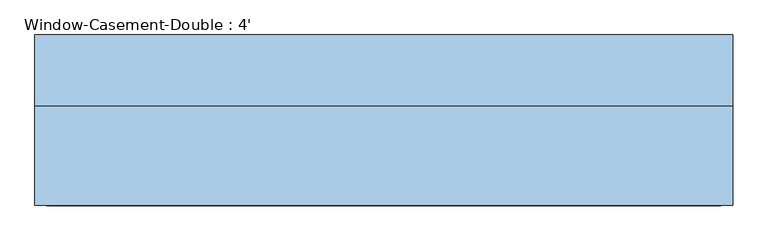
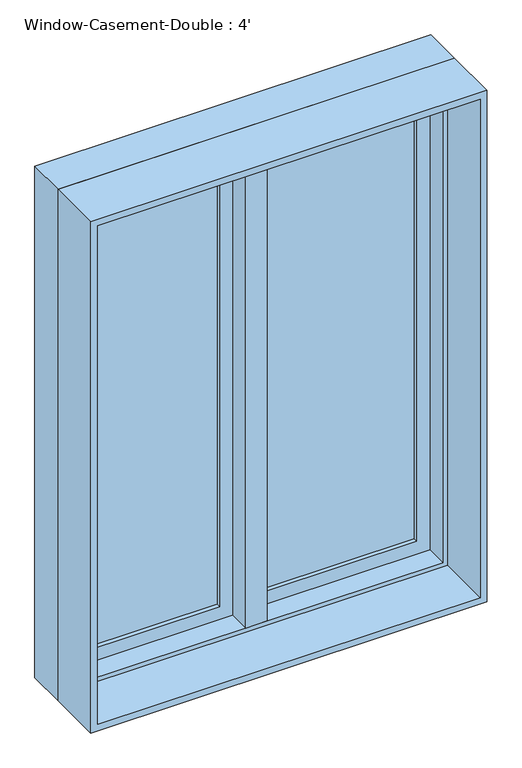
"""IFC4 building model written with IfcOpenShell, lengths in millimetres: window geometry, Window-Casement-Double : 4'."""

from ifc_helpers import new_model, si_unit, frame, origin, place, context, project, spatial, polyline, outline, extrude, faceted_brep, source, transform, mapped, element, save


def window_casement_double_4_9278a0c7(model_context):
    return source(origin(), model_context, "Body", "SolidModel", [
        faceted_brep([(9.525, 146.05, 2425.7), (-9.525, 146.05, 2425.7), (-9.525, 95.25, 2425.7), (9.525, 95.25, 2425.7), (9.525, 146.05, 927.1), (9.525, 95.25, 927.1), (-9.525, 95.25, 927.1), (-9.525, 146.05, 927.1), (-9.525, 95.25, 946.15), (-9.525, 95.25, 2406.65), (-30.1625, 95.25, 946.15), (-30.1625, 95.25, 2406.65), (-30.1625, 31.75, 946.15), (-30.1625, 31.75, 2406.65), (30.1625, 31.75, 946.15), (30.1625, 31.75, 2406.65), (30.1625, 95.25, 946.15), (30.1625, 95.25, 2406.65), (9.525, 95.25, 946.15), (9.525, 95.25, 2406.65)], [[[0, 1, 2, 3]], [[4, 5, 6, 7]], [[1, 0, 4, 7]], [[2, 1, 7, 6, 8, 9]], [[9, 8, 10, 11]], [[11, 10, 12, 13]], [[13, 12, 14, 15]], [[15, 14, 16, 17]], [[17, 16, 18, 19]], [[0, 3, 19, 18, 5, 4]], [[18, 8, 6, 5]], [[9, 19, 3, 2]], [[8, 18, 16, 14, 12, 10]], [[19, 9, 11, 13, 15, 17]]]),
        extrude(outline(polyline([(-66.675, 127.0), (-66.675, 120.65), (-488.95, 120.65), (-488.95, 127.0), (-66.675, 127.0)])), frame((0.0, 0.0, 984.25), z_axis=(0.0, 0.0, 1.0), x_axis=(1.0, 0.0, 0.0)), (0.0, 0.0, 1.0), 1384.3),
        extrude(outline(polyline([(-488.95, 107.95), (-488.95, 114.3), (-66.675, 114.3), (-66.675, 107.95), (-488.95, 107.95)])), frame((0.0, 0.0, 984.25), z_axis=(0.0, 0.0, 1.0), x_axis=(1.0, 0.0, 0.0)), (0.0, 0.0, 1.0), 1384.3),
        extrude(outline(polyline([(488.95, 127.0), (488.95, 120.65), (66.675, 120.65), (66.675, 127.0), (488.95, 127.0)])), frame((0.0, 0.0, 984.25), z_axis=(0.0, 0.0, 1.0), x_axis=(1.0, 0.0, 0.0)), (0.0, 0.0, 1.0), 1384.3),
        extrude(outline(polyline([(66.675, 107.95), (66.675, 114.3), (488.95, 114.3), (488.95, 107.95), (66.675, 107.95)])), frame((0.0, 0.0, 984.25), z_axis=(0.0, 0.0, 1.0), x_axis=(1.0, 0.0, 0.0)), (0.0, 0.0, 1.0), 1384.3),
        extrude(outline(polyline([(2425.7, -546.1), (927.1, -546.1), (927.1, -9.525), (2425.7, -9.525), (2425.7, -546.1)]), holes=[polyline([(2368.55, -66.675), (984.25, -66.675), (984.25, -488.95), (2368.55, -488.95), (2368.55, -66.675)])]), frame((0.0, 95.25, 0.0), z_axis=(0.0, 1.0, 0.0), x_axis=(0.0, 0.0, 1.0)), (0.0, 0.0, 1.0), 44.45),
        extrude(outline(polyline([(927.1, 546.1), (2425.7, 546.1), (2425.7, 9.525), (927.1, 9.525), (927.1, 546.1)]), holes=[polyline([(984.25, 66.675), (2368.55, 66.675), (2368.55, 488.95), (984.25, 488.95), (984.25, 66.675)])]), frame((0.0, 95.25, 0.0), z_axis=(0.0, 1.0, 0.0), x_axis=(0.0, 0.0, 1.0)), (0.0, 0.0, 1.0), 44.45),
        extrude(outline(polyline([(2438.4, -558.8), (914.4, -558.8), (914.4, 558.8), (2438.4, 558.8), (2438.4, -558.8)]), holes=[polyline([(2419.35, 539.75), (933.45, 539.75), (933.45, -539.75), (2419.35, -539.75), (2419.35, 539.75)])]), frame((0.0, -127.0, 0.0), z_axis=(0.0, 1.0, 0.0), x_axis=(0.0, 0.0, 1.0)), (0.0, 0.0, 1.0), 158.75),
        faceted_brep([(527.05, 95.25, 2406.65), (527.05, 31.75, 2406.65), (-527.05, 31.75, 2406.65), (-527.05, 95.25, 2406.65), (546.1, 146.05, 2425.7), (546.1, 95.25, 2425.7), (-546.1, 95.25, 2425.7), (-546.1, 146.05, 2425.7), (558.8, 31.75, 2438.4), (558.8, 146.05, 2438.4), (-558.8, 146.05, 2438.4), (-558.8, 31.75, 2438.4), (-527.05, 31.75, 946.15), (-527.05, 95.25, 946.15), (-546.1, 95.25, 927.1), (-546.1, 146.05, 927.1), (-558.8, 146.05, 914.4), (-558.8, 31.75, 914.4), (527.05, 31.75, 946.15), (527.05, 95.25, 946.15), (546.1, 95.25, 927.1), (546.1, 146.05, 927.1), (558.8, 146.05, 914.4), (558.8, 31.75, 914.4)], [[[0, 1, 2, 3]], [[4, 5, 6, 7]], [[8, 9, 10, 11]], [[3, 2, 12, 13]], [[7, 6, 14, 15]], [[11, 10, 16, 17]], [[13, 12, 18, 19]], [[15, 14, 20, 21]], [[17, 16, 22, 23]], [[11, 17, 23, 8], [1, 18, 12, 2]], [[19, 18, 1, 0]], [[5, 20, 14, 6], [3, 13, 19, 0]], [[21, 20, 5, 4]], [[23, 22, 9, 8]], [[9, 22, 16, 10], [7, 15, 21, 4]]]),
    ])


if __name__ == "__main__":
    model = new_model("IFC4")
    model_context = context("Model", 3, world=origin())
    ifc_project = project(units=[si_unit("LENGTHUNIT", "METRE", prefix="MILLI")], contexts=[model_context])
    site = spatial("IfcSite", under=ifc_project)
    building = spatial("IfcBuilding", under=site)
    placement = place(None, origin())
    window_casement_double_4_shape = window_casement_double_4_9278a0c7(model_context)
    element("IfcWindow", 1, ObjectType="Window-Casement-Double : 4'", at=placement, inside=building, context=model_context, shape_type="MappedRepresentation", body=[
        mapped(window_casement_double_4_shape, transform((0.0, 0.0, 0.0), x_axis=(1.0, 0.0, 0.0), y_axis=(0.0, 1.0, 0.0), z_axis=(0.0, 0.0, 1.0))),
    ])
    save(model, "model.ifc")

# Revit data of these elements
# Type "Window-Casement-Double : 4'"
#   Type Mark = "18"
#   Fire Rating = "0.5h"
#   Assembly Code = "B2020100"
#   Analytic Construction = "Double glazing - domestic"
#   Frame Extension [instance default] = 0' - 0 1/4"
#   Window Inset [instance default] = 0' - 0"
#   Wall Thickness [instance default] = 0' - 6"
#   Interior Wall Closure [instance default] = 0' - 2 1/4"
#   Half Width = 1' - 10"
#   Visual Light Transmittance = 0.81
#   Thermal Resistance (R) = 1.8146 (h·ft²·°F)/BTU
#   Solar Heat Gain Coefficient = 0.76
#   Rough Width = 3' - 8 1/2"
#   Rough Height = 5' - 0 1/2"
#   Height = 5' - 0"
#   Heat Transfer Coefficient (U) = 0.5511 BTU/(h·ft²·°F)
#   Exterior Wall Closure [instance default] = 0' - 1 1/4"
#   Extension Jamb [instance default] = 0' - 2 1/4"
#   Default Sill Height = 3' - 0"
#   Width = 3' - 8"
#   Muntin Visibility = yes
#   Interior Trim Visibility [instance default] = yes
#   Exterior Trim Visibility [instance default] = yes
#   Extension Jamb Visibility [instance default] = yes
#   Interior Trim Material = Wood - Stained
#   Muntin Pattern = Muntin Pattern_2x2 : Muntin Pattern_2x2
#   Interior Trim = Trim-Window-Interior-Flat : Picture Frame
#   Interior Frame Material = Wood - Stained
#   Glass Panel Material = Glass
#   Exterior Trim Material = Clad - White
#   Exterior Trim = Trim-Window-Exterior-Flat : with Sill
#   Exterior Frame Material = Clad - White
#   Wall Closure = (empty or 0)
# Element 1 (IfcWindow, "Window-Casement-Double : 4'")
#   Wall Thickness = 0' - 10"
#   Extension Jamb = 0' - 6 1/4"
#   Materials on its faces: "Wood - Stained", "Glass", "Clad - White"
# Materials
#   "Wood - Stained": class "Wood", colour RGB 224 178 126, transparency 0, Cost = 0
#   "Glass": class "Glass", colour RGB 0 128 192, transparency 0.75, Description = "Soda Lime Glass", Cost = 0
#   "Clad - White": class "Wood", colour RGB 242 242 238, transparency 0, Cost = 0
